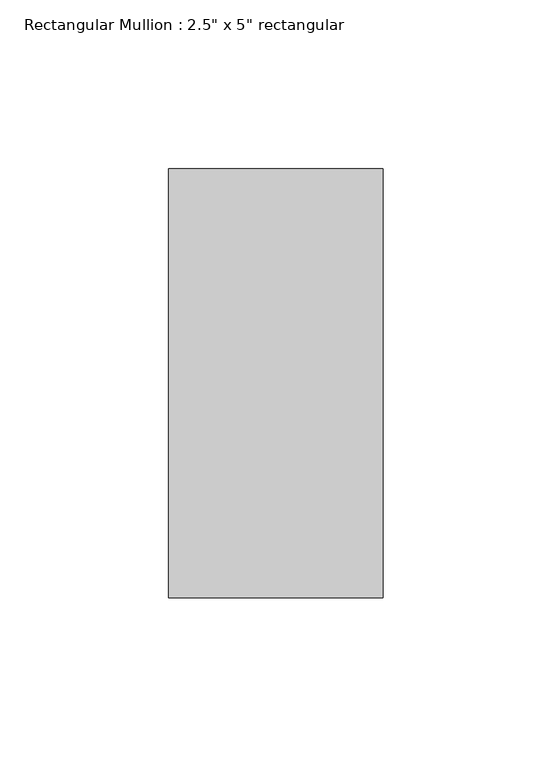
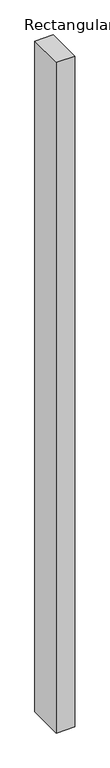
"""IFC4 building model written with IfcOpenShell, lengths in millimetres: member geometry."""

from ifc_helpers import new_model, si_unit, frame, origin, place, context, project, spatial, polyline, outline, extrude, source, transform, mapped, element, save


def member_ee409385(model_context):
    return source(origin(), model_context, "Body", "SweptSolid", [
        extrude(outline(polyline([(0.0, 63.5), (0.0, -63.5), (-63.5, -63.5), (-63.5, 63.5), (0.0, 63.5)])), frame((0.0, 0.0, -2438.4), z_axis=(0.0, 0.0, 1.0), x_axis=(1.0, 0.0, 0.0)), (0.0, 0.0, 1.0), 2438.4),
    ])


if __name__ == "__main__":
    model = new_model("IFC4")
    model_context = context("Model", 3, world=origin())
    ifc_project = project(units=[si_unit("LENGTHUNIT", "METRE", prefix="MILLI")], contexts=[model_context])
    site = spatial("IfcSite", under=ifc_project)
    building = spatial("IfcBuilding", under=site)
    placement = place(None, origin())
    member_shape = member_ee409385(model_context)
    element("IfcMember", 1, ObjectType="Rectangular Mullion : 2.5\" x 5\" rectangular", at=placement, inside=building, context=model_context, shape_type="MappedRepresentation", body=[
        mapped(member_shape, transform((0.0, 0.0, 0.0), x_axis=(1.0, 0.0, 0.0), y_axis=(0.0, 1.0, 0.0), z_axis=(0.0, 0.0, 1.0))),
    ])
    save(model, "model.ifc")

# Revit data of these elements
# Type "Rectangular Mullion : 2.5\" x 5\" rectangular"
#   built-in parameter 1007304 = 0.416667 (stored number, unit not read)
#   built-in parameter 1007301 = 0.104167 (stored number, unit not read)
#   built-in parameter 1007300 = 0.104167 (stored number, unit not read)
